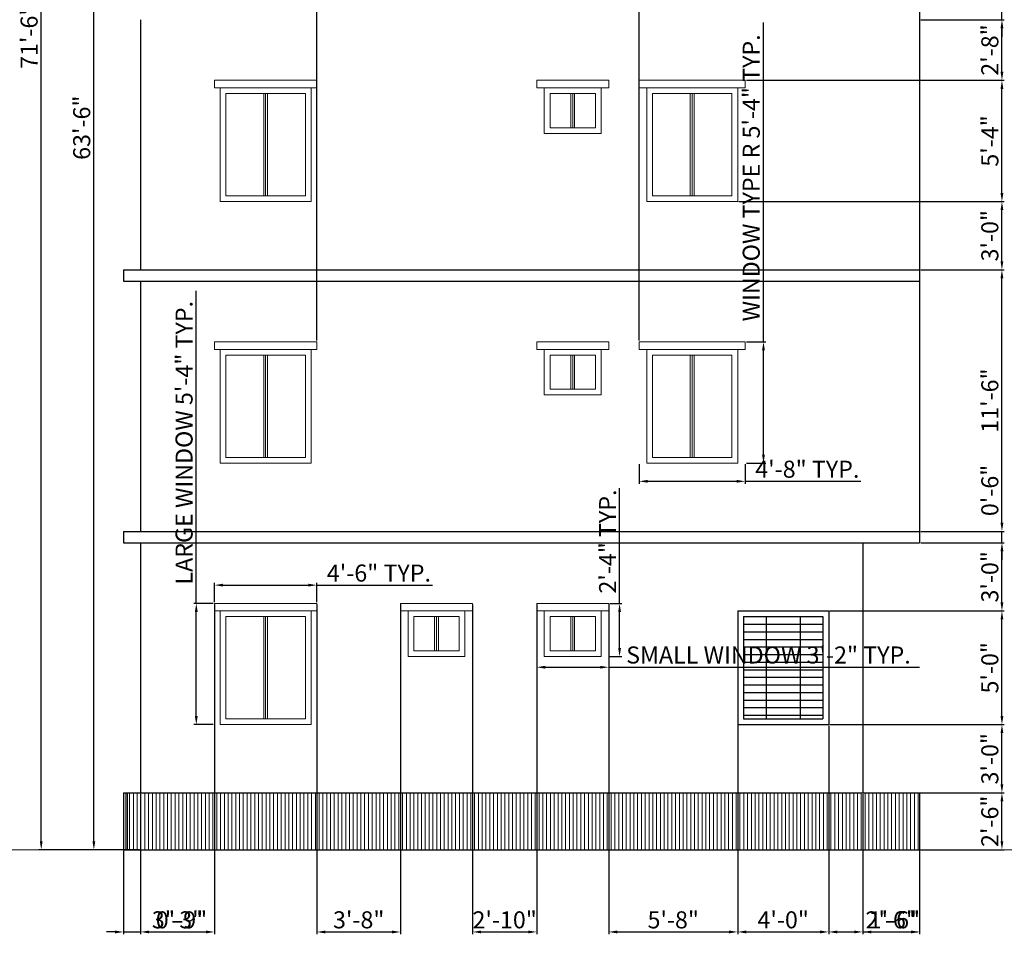
# Model space of a CAD drawing. Units: inches. Extents: x 1692 to 2762, y 798 to 1757.
# Tile 1 of 4: x 1692 to 2211, y 800 to 1282. Entities that reach past the tile are written whole.
import ezdxf

# ---------------------------------------------------------------- set-up
doc = ezdxf.new("R2010")
doc.units = ezdxf.units.IN
for name, color, linetype, lineweight in [('A-ANNO-DIMS', 2, 'Continuous', 18), ('A-CONS', 9, 'Continuous', 13), ('A-ELEV', 7, 'Continuous', 25), ('A-ELEV-PATT', 8, 'Continuous', 13), ('A-GLAZ', 4, 'Continuous', 18)]:
    doc.layers.add(name, color=color, linetype=linetype, lineweight=lineweight)
doc.styles.get("Standard").update_dxf_attribs({"font": 'arial.ttf'})
doc.dimstyles.new('ISO-25', dxfattribs={"dimtxt": 9, "dimasz": 4.5, "dimexe": 1.25, "dimexo": 0.625, "dimtad": 1, "dimdec": 0, "dimlunit": 3, "dimtxsty": 'Standard', "dimcen": 2.5, "dimadec": 0, "dimazin": 0, "dimtfac": 1, "dimtdec": 0, "dimtmove": 0, "dimatfit": 3, "dimfxl": 1, "dimarcsym": 0})

# ---------------------------------------------------------------- blocks, each defined once
blk = doc.blocks.new('*D12')
at = {"layer": 'A-ANNO-DIMS', "color": 0, "lineweight": -2, "transparency": 16777216}
for p, q in [((1755.16, 1606.43), (1729.9, 1606.43)), ((1731.15, 848.93), (1731.15, 1601.93)), ((1755.16, 844.43), (1729.9, 844.43))]:
    blk.add_line(p, q, dxfattribs=at)
at = {"layer": 'A-ANNO-DIMS', "color": 0, "lineweight": 0, "transparency": 16777216}
for points in [[(1730.4, 1601.93), (1731.9, 1601.93), (1731.15, 1606.43)], [(1730.4, 848.93), (1731.9, 848.93), (1731.15, 844.43)]]:
    blk.add_solid(points, dxfattribs=at)
at = {"layer": 'Defpoints', "color": 0, "lineweight": 0, "transparency": 16777216}
for p in [(1731.15, 1606.43), (1755.78, 1606.43), (1755.78, 844.43)]:
    blk.add_point(p, dxfattribs=at)
at = {"layer": 'A-ANNO-DIMS', "color": 0, "transparency": 16777216, "insert": (1725.92, 1225.43), "char_height": 9, "attachment_point": 5, "rotation": 90}
blk.add_mtext('63\'-6"', dxfattribs=at)
blk = doc.blocks.new('WIN-ELEV-L')
for p, q in [((1794.78, 974.43), (1848.78, 974.43)), ((1794.78, 974.43), (1794.78, 970.43)), ((1797.78, 974.43), (1794.78, 974.43)), ((1845.78, 974.43), (1848.78, 974.43)), ((1848.78, 974.43), (1848.78, 970.43)), ((1794.78, 970.43), (1848.78, 970.43)), ((1797.78, 970.43), (1797.78, 910.43)), ((1800.78, 967.43), (1842.78, 967.43)), ((1800.78, 967.43), (1800.78, 913.43)), ((1820.78, 967.43), (1820.78, 913.43)), ((1821.78, 967.43), (1821.78, 913.43)), ((1822.78, 967.43), (1822.78, 913.43)), ((1842.78, 967.43), (1842.78, 913.43)), ((1845.78, 970.43), (1845.78, 910.43)), ((1797.78, 910.43), (1845.78, 910.43)), ((1797.78, 910.43), (1845.78, 910.43)), ((1800.78, 913.43), (1842.78, 913.43))]:
    blk.add_line(p, q)
blk = doc.blocks.new('WIN-ELEV-R')
for p, q in [((2018.78, 1112.43), (2074.78, 1112.43)), ((2018.78, 1112.43), (2018.78, 1108.43)), ((2074.78, 1112.43), (2074.78, 1108.43)), ((2018.78, 1108.43), (2074.78, 1108.43)), ((2022.78, 1108.43), (2022.78, 1048.43)), ((2070.78, 1108.43), (2070.78, 1048.43)), ((2025.78, 1105.43), (2067.78, 1105.43)), ((2025.78, 1105.43), (2025.78, 1051.43)), ((2045.78, 1105.43), (2045.78, 1051.43)), ((2046.78, 1105.43), (2046.78, 1051.43)), ((2047.78, 1105.43), (2047.78, 1051.43)), ((2067.78, 1105.43), (2067.78, 1051.43)), ((2025.78, 1051.43), (2067.78, 1051.43)), ((2022.78, 1048.43), (2070.78, 1048.43))]:
    blk.add_line(p, q)
blk = doc.blocks.new('WIN-ELEV-S')
for p, q in [((1964.78, 974.43), (2002.78, 974.43)), ((1964.78, 974.43), (1964.78, 970.43)), ((2002.78, 974.43), (2002.78, 970.43)), ((1964.78, 970.43), (2002.78, 970.43)), ((1968.78, 970.43), (1968.78, 946.43)), ((1971.78, 967.43), (1995.78, 967.43)), ((1971.78, 967.43), (1971.78, 949.43)), ((1982.78, 967.43), (1982.78, 949.43)), ((1983.78, 967.43), (1983.78, 949.43)), ((1984.78, 967.43), (1984.78, 949.43)), ((1995.78, 967.43), (1995.78, 949.43)), ((1998.78, 970.43), (1998.78, 946.43)), ((1968.78, 946.43), (1998.78, 946.43)), ((1971.78, 949.43), (1995.78, 949.43))]:
    blk.add_line(p, q)
blk = doc.blocks.new('*D18')
at = {"layer": 'A-ANNO-DIMS', "color": 0, "lineweight": -2, "transparency": 16777216}
for p, q in [((1964.78, 945.81), (1964.78, 939.48)), ((2002.78, 945.81), (2002.78, 939.48)), ((1969.28, 940.73), (1998.28, 940.73)), ((2002.78, 940.73), (2166.73, 940.73))]:
    blk.add_line(p, q, dxfattribs=at)
at = {"layer": 'A-ANNO-DIMS', "color": 0, "lineweight": 0, "transparency": 16777216}
for points in [[(1969.28, 941.48), (1969.28, 939.98), (1964.78, 940.73)], [(1998.28, 941.48), (1998.28, 939.98), (2002.78, 940.73)]]:
    blk.add_solid(points, dxfattribs=at)
at = {"layer": 'Defpoints', "color": 0, "lineweight": 0, "transparency": 16777216}
for p in [(1964.78, 946.43), (2002.78, 946.43), (2002.78, 940.73)]:
    blk.add_point(p, dxfattribs=at)
at = {"layer": 'A-ANNO-DIMS', "color": 0, "transparency": 16777216, "insert": (2087.01, 946.02), "char_height": 9, "attachment_point": 5}
blk.add_mtext('SMALL WINDOW 3\'-2" TYP.', dxfattribs=at)
blk = doc.blocks.new('*D19')
at = {"layer": 'A-ANNO-DIMS', "color": 0, "lineweight": -2, "transparency": 16777216}
for p, q in [((2008.48, 974.43), (2008.48, 1035.2)), ((2003.41, 974.43), (2009.73, 974.43)), ((2008.48, 950.93), (2008.48, 969.93)), ((2003.41, 946.43), (2009.73, 946.43))]:
    blk.add_line(p, q, dxfattribs=at)
at = {"layer": 'A-ANNO-DIMS', "color": 0, "lineweight": 0, "transparency": 16777216}
for points in [[(2007.73, 969.93), (2009.23, 969.93), (2008.48, 974.43)], [(2007.73, 950.93), (2009.23, 950.93), (2008.48, 946.43)]]:
    blk.add_solid(points, dxfattribs=at)
at = {"layer": 'Defpoints', "color": 0, "lineweight": 0, "transparency": 16777216}
for p in [(2002.78, 974.43), (2008.48, 974.43), (2002.78, 946.43)]:
    blk.add_point(p, dxfattribs=at)
at = {"layer": 'A-ANNO-DIMS', "color": 0, "transparency": 16777216, "insert": (2003.33, 1007.06), "char_height": 9, "attachment_point": 5, "rotation": 90}
blk.add_mtext('2\'-4" TYP.', dxfattribs=at)
blk = doc.blocks.new('*D20')
at = {"layer": 'A-ANNO-DIMS', "color": 0, "lineweight": -2, "transparency": 16777216}
for p, q in [((1785.18, 974.43), (1785.18, 1139.42)), ((1794.16, 974.43), (1783.93, 974.43)), ((1785.18, 914.93), (1785.18, 969.93)), ((1794.16, 910.43), (1783.93, 910.43))]:
    blk.add_line(p, q, dxfattribs=at)
at = {"layer": 'A-ANNO-DIMS', "color": 0, "lineweight": 0, "transparency": 16777216}
for points in [[(1784.43, 969.93), (1785.93, 969.93), (1785.18, 974.43)], [(1784.43, 914.93), (1785.93, 914.93), (1785.18, 910.43)]]:
    blk.add_solid(points, dxfattribs=at)
at = {"layer": 'Defpoints', "color": 0, "lineweight": 0, "transparency": 16777216}
for p in [(1785.18, 974.43), (1794.78, 974.43), (1794.78, 910.43)]:
    blk.add_point(p, dxfattribs=at)
at = {"layer": 'A-ANNO-DIMS', "color": 0, "transparency": 16777216, "insert": (1779.9, 1059.18), "char_height": 9, "attachment_point": 5, "rotation": 90}
blk.add_mtext('LARGE WINDOW 5\'-4" TYP.', dxfattribs=at)
blk = doc.blocks.new('*D21')
at = {"layer": 'A-ANNO-DIMS', "color": 0, "lineweight": -2, "transparency": 16777216}
for p, q in [((1794.78, 975.06), (1794.78, 985.28)), ((1799.28, 984.03), (1844.28, 984.03)), ((1848.78, 975.06), (1848.78, 985.28)), ((1848.78, 984.03), (1909.75, 984.03))]:
    blk.add_line(p, q, dxfattribs=at)
at = {"layer": 'A-ANNO-DIMS', "color": 0, "lineweight": 0, "transparency": 16777216}
for points in [[(1799.28, 984.78), (1799.28, 983.28), (1794.78, 984.03)], [(1844.28, 984.78), (1844.28, 983.28), (1848.78, 984.03)]]:
    blk.add_solid(points, dxfattribs=at)
at = {"layer": 'Defpoints', "color": 0, "lineweight": 0, "transparency": 16777216}
for p in [(1848.78, 984.03), (1794.78, 974.43), (1848.78, 974.43)]:
    blk.add_point(p, dxfattribs=at)
at = {"layer": 'A-ANNO-DIMS', "color": 0, "transparency": 16777216, "insert": (1881.52, 989.25), "char_height": 9, "attachment_point": 5}
blk.add_mtext('4\'-6" TYP.', dxfattribs=at)
blk = doc.blocks.new('*D22')
at = {"layer": 'A-ANNO-DIMS', "color": 0, "lineweight": -2, "transparency": 16777216}
for p, q in [((2084.38, 1112.43), (2084.38, 1280.97)), ((2075.41, 1112.43), (2085.63, 1112.43)), ((2084.38, 1052.93), (2084.38, 1107.93)), ((2075.41, 1048.43), (2085.63, 1048.43))]:
    blk.add_line(p, q, dxfattribs=at)
at = {"layer": 'A-ANNO-DIMS', "color": 0, "lineweight": 0, "transparency": 16777216}
for points in [[(2083.63, 1107.93), (2085.13, 1107.93), (2084.38, 1112.43)], [(2083.63, 1052.93), (2085.13, 1052.93), (2084.38, 1048.43)]]:
    blk.add_solid(points, dxfattribs=at)
at = {"layer": 'Defpoints', "color": 0, "lineweight": 0, "transparency": 16777216}
for p in [(2074.78, 1112.43), (2084.38, 1112.43), (2074.78, 1048.43)]:
    blk.add_point(p, dxfattribs=at)
at = {"layer": 'A-ANNO-DIMS', "color": 0, "transparency": 16777216, "insert": (2079.1, 1198.95), "char_height": 9, "attachment_point": 5, "rotation": 90}
blk.add_mtext('WINDOW TYPE R 5\'-4" TYP.', dxfattribs=at)
blk = doc.blocks.new('*D23')
at = {"layer": 'A-ANNO-DIMS', "color": 0, "lineweight": -2, "transparency": 16777216}
for p, q in [((2018.78, 1047.81), (2018.78, 1037.58)), ((2074.78, 1047.81), (2074.78, 1037.58)), ((2023.28, 1038.83), (2070.28, 1038.83)), ((2074.78, 1038.83), (2135.75, 1038.83))]:
    blk.add_line(p, q, dxfattribs=at)
at = {"layer": 'A-ANNO-DIMS', "color": 0, "lineweight": 0, "transparency": 16777216}
for points in [[(2023.28, 1039.58), (2023.28, 1038.08), (2018.78, 1038.83)], [(2070.28, 1039.58), (2070.28, 1038.08), (2074.78, 1038.83)]]:
    blk.add_solid(points, dxfattribs=at)
at = {"layer": 'Defpoints', "color": 0, "lineweight": 0, "transparency": 16777216}
for p in [(2018.78, 1048.43), (2074.78, 1048.43), (2074.78, 1038.83)]:
    blk.add_point(p, dxfattribs=at)
at = {"layer": 'A-ANNO-DIMS', "color": 0, "transparency": 16777216, "insert": (2107.52, 1044.05), "char_height": 9, "attachment_point": 5}
blk.add_mtext('4\'-8" TYP.', dxfattribs=at)
blk = doc.blocks.new('*D24')
at = {"layer": 'A-ANNO-DIMS', "color": 0, "lineweight": -2, "transparency": 16777216}
for p, q in [((1950.16, 1702.43), (1702.13, 1702.43)), ((1703.38, 848.93), (1703.38, 1697.93)), ((1746.16, 844.43), (1702.13, 844.43))]:
    blk.add_line(p, q, dxfattribs=at)
at = {"layer": 'A-ANNO-DIMS', "color": 0, "lineweight": 0, "transparency": 16777216}
for points in [[(1702.63, 1697.93), (1704.13, 1697.93), (1703.38, 1702.43)], [(1702.63, 848.93), (1704.13, 848.93), (1703.38, 844.43)]]:
    blk.add_solid(points, dxfattribs=at)
at = {"layer": 'Defpoints', "color": 0, "lineweight": 0, "transparency": 16777216}
for p in [(1703.38, 1702.43), (1950.78, 1702.43), (1746.78, 844.43)]:
    blk.add_point(p, dxfattribs=at)
at = {"layer": 'A-ANNO-DIMS', "color": 0, "transparency": 16777216, "insert": (1698.16, 1273.43), "char_height": 9, "attachment_point": 5, "rotation": 90}
blk.add_mtext('71\'-6"', dxfattribs=at)
blk = doc.blocks.new('*D25')
at = {"layer": 'A-ANNO-DIMS', "color": 0, "lineweight": -2, "transparency": 16777216}
for p, q in [((2167.41, 874.43), (2211.43, 874.43)), ((2210.18, 848.93), (2210.18, 869.93)), ((2167.41, 844.43), (2211.43, 844.43))]:
    blk.add_line(p, q, dxfattribs=at)
at = {"layer": 'A-ANNO-DIMS', "color": 0, "lineweight": 0, "transparency": 16777216}
for points in [[(2209.43, 869.93), (2210.93, 869.93), (2210.18, 874.43)], [(2209.43, 848.93), (2210.93, 848.93), (2210.18, 844.43)]]:
    blk.add_solid(points, dxfattribs=at)
at = {"layer": 'Defpoints', "color": 0, "lineweight": 0, "transparency": 16777216}
for p in [(2166.78, 874.43), (2210.18, 874.43), (2166.78, 844.43)]:
    blk.add_point(p, dxfattribs=at)
at = {"layer": 'A-ANNO-DIMS', "color": 0, "transparency": 16777216, "insert": (2204.96, 859.43), "char_height": 9, "attachment_point": 5, "rotation": 90}
blk.add_mtext('2\'-6"', dxfattribs=at)
blk = doc.blocks.new('*D26')
at = {"layer": 'A-ANNO-DIMS', "color": 0, "lineweight": -2, "transparency": 16777216}
for p, q in [((2119.41, 910.43), (2211.43, 910.43)), ((2210.18, 878.93), (2210.18, 905.93)), ((2137.41, 874.43), (2211.43, 874.43))]:
    blk.add_line(p, q, dxfattribs=at)
at = {"layer": 'A-ANNO-DIMS', "color": 0, "lineweight": 0, "transparency": 16777216}
for points in [[(2209.43, 905.93), (2210.93, 905.93), (2210.18, 910.43)], [(2209.43, 878.93), (2210.93, 878.93), (2210.18, 874.43)]]:
    blk.add_solid(points, dxfattribs=at)
at = {"layer": 'Defpoints', "color": 0, "lineweight": 0, "transparency": 16777216}
for p in [(2118.78, 910.43), (2210.18, 910.43), (2136.78, 874.43)]:
    blk.add_point(p, dxfattribs=at)
at = {"layer": 'A-ANNO-DIMS', "color": 0, "transparency": 16777216, "insert": (2204.96, 892.43), "char_height": 9, "attachment_point": 5, "rotation": 90}
blk.add_mtext('3\'-0"', dxfattribs=at)
blk = doc.blocks.new('*D27')
at = {"layer": 'A-ANNO-DIMS', "color": 0, "lineweight": -2, "transparency": 16777216}
for p, q in [((2119.41, 970.43), (2211.43, 970.43)), ((2210.18, 914.93), (2210.18, 965.93)), ((2119.41, 910.43), (2211.43, 910.43))]:
    blk.add_line(p, q, dxfattribs=at)
at = {"layer": 'A-ANNO-DIMS', "color": 0, "lineweight": 0, "transparency": 16777216}
for points in [[(2209.43, 965.93), (2210.93, 965.93), (2210.18, 970.43)], [(2209.43, 914.93), (2210.93, 914.93), (2210.18, 910.43)]]:
    blk.add_solid(points, dxfattribs=at)
at = {"layer": 'Defpoints', "color": 0, "lineweight": 0, "transparency": 16777216}
for p in [(2118.78, 970.43), (2210.18, 970.43), (2118.78, 910.43)]:
    blk.add_point(p, dxfattribs=at)
at = {"layer": 'A-ANNO-DIMS', "color": 0, "transparency": 16777216, "insert": (2204.96, 940.43), "char_height": 9, "attachment_point": 5, "rotation": 90}
blk.add_mtext('5\'-0"', dxfattribs=at)
blk = doc.blocks.new('*D28')
at = {"layer": 'A-ANNO-DIMS', "color": 0, "lineweight": -2, "transparency": 16777216}
for p, q in [((2167.41, 1006.43), (2211.43, 1006.43)), ((2210.18, 974.93), (2210.18, 1001.93)), ((2119.41, 970.43), (2211.43, 970.43))]:
    blk.add_line(p, q, dxfattribs=at)
at = {"layer": 'A-ANNO-DIMS', "color": 0, "lineweight": 0, "transparency": 16777216}
for points in [[(2209.43, 1001.93), (2210.93, 1001.93), (2210.18, 1006.43)], [(2209.43, 974.93), (2210.93, 974.93), (2210.18, 970.43)]]:
    blk.add_solid(points, dxfattribs=at)
at = {"layer": 'Defpoints', "color": 0, "lineweight": 0, "transparency": 16777216}
for p in [(2166.78, 1006.43), (2210.18, 1006.43), (2118.78, 970.43)]:
    blk.add_point(p, dxfattribs=at)
at = {"layer": 'A-ANNO-DIMS', "color": 0, "transparency": 16777216, "insert": (2204.96, 988.43), "char_height": 9, "attachment_point": 5, "rotation": 90}
blk.add_mtext('3\'-0"', dxfattribs=at)
blk = doc.blocks.new('*D29')
at = {"layer": 'A-ANNO-DIMS', "color": 0, "lineweight": -2, "transparency": 16777216}
for p, q in [((2210.18, 1016.93), (2210.18, 1046.61)), ((2167.41, 1012.43), (2211.43, 1012.43)), ((2210.18, 1006.43), (2210.18, 1012.43)), ((2167.41, 1006.43), (2211.43, 1006.43)), ((2210.18, 1001.93), (2210.18, 997.43))]:
    blk.add_line(p, q, dxfattribs=at)
at = {"layer": 'A-ANNO-DIMS', "color": 0, "lineweight": 0, "transparency": 16777216}
for points in [[(2209.43, 1016.93), (2210.93, 1016.93), (2210.18, 1012.43)], [(2209.43, 1001.93), (2210.93, 1001.93), (2210.18, 1006.43)]]:
    blk.add_solid(points, dxfattribs=at)
at = {"layer": 'Defpoints', "color": 0, "lineweight": 0, "transparency": 16777216}
for p in [(2166.78, 1012.43), (2210.18, 1012.43), (2166.78, 1006.43)]:
    blk.add_point(p, dxfattribs=at)
at = {"layer": 'A-ANNO-DIMS', "color": 0, "transparency": 16777216, "insert": (2204.96, 1034.02), "char_height": 9, "attachment_point": 5, "rotation": 90}
blk.add_mtext('0\'-6"', dxfattribs=at)
blk = doc.blocks.new('*D30')
at = {"layer": 'A-ANNO-DIMS', "color": 0, "lineweight": -2, "transparency": 16777216}
for p, q in [((2167.41, 1150.43), (2211.43, 1150.43)), ((2210.18, 1016.93), (2210.18, 1145.93)), ((2167.41, 1012.43), (2211.43, 1012.43))]:
    blk.add_line(p, q, dxfattribs=at)
at = {"layer": 'A-ANNO-DIMS', "color": 0, "lineweight": 0, "transparency": 16777216}
for points in [[(2209.43, 1145.93), (2210.93, 1145.93), (2210.18, 1150.43)], [(2209.43, 1016.93), (2210.93, 1016.93), (2210.18, 1012.43)]]:
    blk.add_solid(points, dxfattribs=at)
at = {"layer": 'Defpoints', "color": 0, "lineweight": 0, "transparency": 16777216}
for p in [(2166.78, 1150.43), (2210.18, 1150.43), (2166.78, 1012.43)]:
    blk.add_point(p, dxfattribs=at)
at = {"layer": 'A-ANNO-DIMS', "color": 0, "transparency": 16777216, "insert": (2204.96, 1081.43), "char_height": 9, "attachment_point": 5, "rotation": 90}
blk.add_mtext('11\'-6"', dxfattribs=at)
blk = doc.blocks.new('*D31')
at = {"layer": 'A-ANNO-DIMS', "color": 0, "lineweight": -2, "transparency": 16777216}
for p, q in [((2071.41, 1186.43), (2211.43, 1186.43)), ((2210.18, 1154.93), (2210.18, 1181.93)), ((2167.41, 1150.43), (2211.43, 1150.43))]:
    blk.add_line(p, q, dxfattribs=at)
at = {"layer": 'A-ANNO-DIMS', "color": 0, "lineweight": 0, "transparency": 16777216}
for points in [[(2209.43, 1181.93), (2210.93, 1181.93), (2210.18, 1186.43)], [(2209.43, 1154.93), (2210.93, 1154.93), (2210.18, 1150.43)]]:
    blk.add_solid(points, dxfattribs=at)
at = {"layer": 'Defpoints', "color": 0, "lineweight": 0, "transparency": 16777216}
for p in [(2070.78, 1186.43), (2210.18, 1186.43), (2166.78, 1150.43)]:
    blk.add_point(p, dxfattribs=at)
at = {"layer": 'A-ANNO-DIMS', "color": 0, "transparency": 16777216, "insert": (2204.96, 1168.43), "char_height": 9, "attachment_point": 5, "rotation": 90}
blk.add_mtext('3\'-0"', dxfattribs=at)
blk = doc.blocks.new('*D32')
at = {"layer": 'A-ANNO-DIMS', "color": 0, "lineweight": -2, "transparency": 16777216}
for p, q in [((2075.41, 1250.43), (2211.43, 1250.43)), ((2210.18, 1190.93), (2210.18, 1245.93)), ((2071.41, 1186.43), (2211.43, 1186.43))]:
    blk.add_line(p, q, dxfattribs=at)
at = {"layer": 'A-ANNO-DIMS', "color": 0, "lineweight": 0, "transparency": 16777216}
for points in [[(2209.43, 1245.93), (2210.93, 1245.93), (2210.18, 1250.43)], [(2209.43, 1190.93), (2210.93, 1190.93), (2210.18, 1186.43)]]:
    blk.add_solid(points, dxfattribs=at)
at = {"layer": 'Defpoints', "color": 0, "lineweight": 0, "transparency": 16777216}
for p in [(2074.78, 1250.43), (2210.18, 1250.43), (2070.78, 1186.43)]:
    blk.add_point(p, dxfattribs=at)
at = {"layer": 'A-ANNO-DIMS', "color": 0, "transparency": 16777216, "insert": (2204.98, 1218.43), "char_height": 9, "attachment_point": 5, "rotation": 90}
blk.add_mtext('5\'-4"', dxfattribs=at)
blk = doc.blocks.new('*D33')
at = {"layer": 'A-ANNO-DIMS', "color": 0, "lineweight": -2, "transparency": 16777216}
for p, q in [((2167.41, 1282.43), (2211.43, 1282.43)), ((2210.18, 1254.93), (2210.18, 1277.93)), ((2075.41, 1250.43), (2211.43, 1250.43))]:
    blk.add_line(p, q, dxfattribs=at)
at = {"layer": 'A-ANNO-DIMS', "color": 0, "lineweight": 0, "transparency": 16777216}
for points in [[(2209.43, 1277.93), (2210.93, 1277.93), (2210.18, 1282.43)], [(2209.43, 1254.93), (2210.93, 1254.93), (2210.18, 1250.43)]]:
    blk.add_solid(points, dxfattribs=at)
at = {"layer": 'Defpoints', "color": 0, "lineweight": 0, "transparency": 16777216}
for p in [(2166.78, 1282.43), (2210.18, 1282.43), (2074.78, 1250.43)]:
    blk.add_point(p, dxfattribs=at)
at = {"layer": 'A-ANNO-DIMS', "color": 0, "transparency": 16777216, "insert": (2204.96, 1266.43), "char_height": 9, "attachment_point": 5, "rotation": 90}
blk.add_mtext('2\'-8"', dxfattribs=at)
blk = doc.blocks.new('*D34')
at = {"layer": 'A-ANNO-DIMS', "color": 0, "lineweight": -2, "transparency": 16777216}
for p, q in [((2210.18, 1292.93), (2210.18, 1322.61)), ((2167.41, 1288.43), (2211.43, 1288.43)), ((2210.18, 1282.43), (2210.18, 1288.43)), ((2167.41, 1282.43), (2211.43, 1282.43)), ((2210.18, 1277.93), (2210.18, 1273.43))]:
    blk.add_line(p, q, dxfattribs=at)
at = {"layer": 'A-ANNO-DIMS', "color": 0, "lineweight": 0, "transparency": 16777216}
for points in [[(2209.43, 1292.93), (2210.93, 1292.93), (2210.18, 1288.43)], [(2209.43, 1277.93), (2210.93, 1277.93), (2210.18, 1282.43)]]:
    blk.add_solid(points, dxfattribs=at)
at = {"layer": 'Defpoints', "color": 0, "lineweight": 0, "transparency": 16777216}
for p in [(2166.78, 1288.43), (2210.18, 1288.43), (2166.78, 1282.43)]:
    blk.add_point(p, dxfattribs=at)
at = {"layer": 'A-ANNO-DIMS', "color": 0, "transparency": 16777216, "insert": (2204.96, 1310.02), "char_height": 9, "attachment_point": 5, "rotation": 90}
blk.add_mtext('0\'-6"', dxfattribs=at)
blk = doc.blocks.new('*D39')
at = {"layer": 'A-ANNO-DIMS', "color": 0, "lineweight": -2, "transparency": 16777216}
for p, q in [((1755.78, 873.81), (1755.78, 799.78)), ((1746.78, 843.81), (1746.78, 799.78)), ((1742.28, 801.03), (1737.78, 801.03)), ((1746.78, 801.03), (1755.78, 801.03)), ((1760.28, 801.03), (1789.95, 801.03))]:
    blk.add_line(p, q, dxfattribs=at)
at = {"layer": 'A-ANNO-DIMS', "color": 0, "lineweight": 0, "transparency": 16777216}
for points in [[(1742.28, 801.78), (1742.28, 800.28), (1746.78, 801.03)], [(1760.28, 801.78), (1760.28, 800.28), (1755.78, 801.03)]]:
    blk.add_solid(points, dxfattribs=at)
at = {"layer": 'Defpoints', "color": 0, "lineweight": 0, "transparency": 16777216}
for p in [(1755.78, 874.43), (1746.78, 844.43), (1755.78, 801.03)]:
    blk.add_point(p, dxfattribs=at)
at = {"layer": 'A-ANNO-DIMS', "color": 0, "transparency": 16777216, "insert": (1777.37, 806.25), "char_height": 9, "attachment_point": 5}
blk.add_mtext('0\'-9"', dxfattribs=at)
blk = doc.blocks.new('*D40')
at = {"layer": 'A-ANNO-DIMS', "color": 0, "lineweight": -2, "transparency": 16777216}
for p, q in [((1794.78, 973.81), (1794.78, 799.78)), ((1755.78, 873.81), (1755.78, 799.78)), ((1760.28, 801.03), (1790.28, 801.03))]:
    blk.add_line(p, q, dxfattribs=at)
at = {"layer": 'A-ANNO-DIMS', "color": 0, "lineweight": 0, "transparency": 16777216}
for points in [[(1760.28, 801.78), (1760.28, 800.28), (1755.78, 801.03)], [(1790.28, 801.78), (1790.28, 800.28), (1794.78, 801.03)]]:
    blk.add_solid(points, dxfattribs=at)
at = {"layer": 'Defpoints', "color": 0, "lineweight": 0, "transparency": 16777216}
for p in [(1794.78, 974.43), (1755.78, 874.43), (1794.78, 801.03)]:
    blk.add_point(p, dxfattribs=at)
at = {"layer": 'A-ANNO-DIMS', "color": 0, "transparency": 16777216, "insert": (1775.28, 806.26), "char_height": 9, "attachment_point": 5}
blk.add_mtext('3\'-3"', dxfattribs=at)
blk = doc.blocks.new('*D41')
at = {"layer": 'A-ANNO-DIMS', "color": 0, "lineweight": -2, "transparency": 16777216}
for p, q in [((1848.78, 973.81), (1848.78, 799.78)), ((1892.93, 973.81), (1892.93, 799.78)), ((1853.28, 801.03), (1888.43, 801.03))]:
    blk.add_line(p, q, dxfattribs=at)
at = {"layer": 'A-ANNO-DIMS', "color": 0, "lineweight": 0, "transparency": 16777216}
for points in [[(1853.28, 801.78), (1853.28, 800.28), (1848.78, 801.03)], [(1888.43, 801.78), (1888.43, 800.28), (1892.93, 801.03)]]:
    blk.add_solid(points, dxfattribs=at)
at = {"layer": 'Defpoints', "color": 0, "lineweight": 0, "transparency": 16777216}
for p in [(1848.78, 974.43), (1892.93, 974.43), (1892.93, 801.03)]:
    blk.add_point(p, dxfattribs=at)
at = {"layer": 'A-ANNO-DIMS', "color": 0, "transparency": 16777216, "insert": (1870.86, 806.26), "char_height": 9, "attachment_point": 5}
blk.add_mtext('3\'-8"', dxfattribs=at)
blk = doc.blocks.new('*D42')
at = {"layer": 'A-ANNO-DIMS', "color": 0, "lineweight": -2, "transparency": 16777216}
for p, q in [((1930.93, 973.81), (1930.93, 799.78)), ((1964.78, 973.81), (1964.78, 799.78)), ((1935.43, 801.03), (1960.28, 801.03))]:
    blk.add_line(p, q, dxfattribs=at)
at = {"layer": 'A-ANNO-DIMS', "color": 0, "lineweight": 0, "transparency": 16777216}
for points in [[(1935.43, 801.78), (1935.43, 800.28), (1930.93, 801.03)], [(1960.28, 801.78), (1960.28, 800.28), (1964.78, 801.03)]]:
    blk.add_solid(points, dxfattribs=at)
at = {"layer": 'Defpoints', "color": 0, "lineweight": 0, "transparency": 16777216}
for p in [(1930.93, 974.43), (1964.78, 974.43), (1964.78, 801.03)]:
    blk.add_point(p, dxfattribs=at)
at = {"layer": 'A-ANNO-DIMS', "color": 0, "transparency": 16777216, "insert": (1947.86, 806.25), "char_height": 9, "attachment_point": 5}
blk.add_mtext('2\'-10"', dxfattribs=at)
blk = doc.blocks.new('*D43')
at = {"layer": 'A-ANNO-DIMS', "color": 0, "lineweight": -2, "transparency": 16777216}
for p, q in [((2002.78, 973.81), (2002.78, 799.78)), ((2070.78, 969.81), (2070.78, 799.78)), ((2007.28, 801.03), (2066.28, 801.03))]:
    blk.add_line(p, q, dxfattribs=at)
at = {"layer": 'A-ANNO-DIMS', "color": 0, "lineweight": 0, "transparency": 16777216}
for points in [[(2007.28, 801.78), (2007.28, 800.28), (2002.78, 801.03)], [(2066.28, 801.78), (2066.28, 800.28), (2070.78, 801.03)]]:
    blk.add_solid(points, dxfattribs=at)
at = {"layer": 'Defpoints', "color": 0, "lineweight": 0, "transparency": 16777216}
for p in [(2002.78, 974.43), (2070.78, 970.43), (2070.78, 801.03)]:
    blk.add_point(p, dxfattribs=at)
at = {"layer": 'A-ANNO-DIMS', "color": 0, "transparency": 16777216, "insert": (2036.78, 806.25), "char_height": 9, "attachment_point": 5}
blk.add_mtext('5\'-8"', dxfattribs=at)
blk = doc.blocks.new('*D44')
at = {"layer": 'A-ANNO-DIMS', "color": 0, "lineweight": -2, "transparency": 16777216}
for p, q in [((2070.78, 909.81), (2070.78, 799.78)), ((2118.78, 909.81), (2118.78, 799.78)), ((2075.28, 801.03), (2114.28, 801.03))]:
    blk.add_line(p, q, dxfattribs=at)
at = {"layer": 'A-ANNO-DIMS', "color": 0, "lineweight": 0, "transparency": 16777216}
for points in [[(2075.28, 801.78), (2075.28, 800.28), (2070.78, 801.03)], [(2114.28, 801.78), (2114.28, 800.28), (2118.78, 801.03)]]:
    blk.add_solid(points, dxfattribs=at)
at = {"layer": 'Defpoints', "color": 0, "lineweight": 0, "transparency": 16777216}
for p in [(2070.78, 910.43), (2118.78, 910.43), (2118.78, 801.03)]:
    blk.add_point(p, dxfattribs=at)
at = {"layer": 'A-ANNO-DIMS', "color": 0, "transparency": 16777216, "insert": (2094.78, 806.25), "char_height": 9, "attachment_point": 5}
blk.add_mtext('4\'-0"', dxfattribs=at)
blk = doc.blocks.new('*D45')
at = {"layer": 'A-ANNO-DIMS', "color": 0, "lineweight": -2, "transparency": 16777216}
for p, q in [((2118.78, 909.81), (2118.78, 799.78)), ((2136.78, 873.81), (2136.78, 799.78)), ((2123.28, 801.03), (2132.28, 801.03)), ((2136.78, 801.03), (2165.61, 801.03))]:
    blk.add_line(p, q, dxfattribs=at)
at = {"layer": 'A-ANNO-DIMS', "color": 0, "lineweight": 0, "transparency": 16777216}
for points in [[(2123.28, 801.78), (2123.28, 800.28), (2118.78, 801.03)], [(2132.28, 801.78), (2132.28, 800.28), (2136.78, 801.03)]]:
    blk.add_solid(points, dxfattribs=at)
at = {"layer": 'Defpoints', "color": 0, "lineweight": 0, "transparency": 16777216}
for p in [(2118.78, 910.43), (2136.78, 874.43), (2136.78, 801.03)]:
    blk.add_point(p, dxfattribs=at)
at = {"layer": 'A-ANNO-DIMS', "color": 0, "transparency": 16777216, "insert": (2153.44, 806.25), "char_height": 9, "attachment_point": 5}
blk.add_mtext('1\'-6"', dxfattribs=at)
blk = doc.blocks.new('*D46')
at = {"layer": 'A-ANNO-DIMS', "color": 0, "lineweight": -2, "transparency": 16777216}
for p, q in [((2136.78, 873.81), (2136.78, 799.78)), ((2166.78, 873.81), (2166.78, 799.78)), ((2141.28, 801.03), (2162.28, 801.03))]:
    blk.add_line(p, q, dxfattribs=at)
at = {"layer": 'A-ANNO-DIMS', "color": 0, "lineweight": 0, "transparency": 16777216}
for points in [[(2141.28, 801.78), (2141.28, 800.28), (2136.78, 801.03)], [(2162.28, 801.78), (2162.28, 800.28), (2166.78, 801.03)]]:
    blk.add_solid(points, dxfattribs=at)
at = {"layer": 'Defpoints', "color": 0, "lineweight": 0, "transparency": 16777216}
for p in [(2136.78, 874.43), (2166.78, 874.43), (2166.78, 801.03)]:
    blk.add_point(p, dxfattribs=at)
at = {"layer": 'A-ANNO-DIMS', "color": 0, "transparency": 16777216, "insert": (2151.78, 806.25), "char_height": 9, "attachment_point": 5}
blk.add_mtext('2\'-6"', dxfattribs=at)
blk = doc.blocks.new('*D47')
at = {"layer": 'A-ANNO-DIMS', "color": 0, "lineweight": -2, "transparency": 16777216}
for p, q in [((1848.78, 1113.06), (1848.78, 1747.08)), ((1853.28, 1745.83), (2014.28, 1745.83)), ((2018.78, 1113.06), (2018.78, 1747.08))]:
    blk.add_line(p, q, dxfattribs=at)
at = {"layer": 'A-ANNO-DIMS', "color": 0, "lineweight": 0, "transparency": 16777216}
for points in [[(1853.28, 1746.58), (1853.28, 1745.08), (1848.78, 1745.83)], [(2014.28, 1746.58), (2014.28, 1745.08), (2018.78, 1745.83)]]:
    blk.add_solid(points, dxfattribs=at)
at = {"layer": 'Defpoints', "color": 0, "lineweight": 0, "transparency": 16777216}
for p in [(2018.78, 1745.83), (1848.78, 1112.43), (2018.78, 1112.43)]:
    blk.add_point(p, dxfattribs=at)
at = {"layer": 'A-ANNO-DIMS', "color": 0, "transparency": 16777216, "insert": (1933.78, 1750.98), "char_height": 9, "attachment_point": 5}
blk.add_mtext('14\'-2"', dxfattribs=at)

msp = doc.modelspace()

# ---------------------------------------------------------------- hatches: boundary and pattern name
at = {"layer": 'A-ELEV-PATT'}
h = msp.add_hatch(dxfattribs=at)
h.set_pattern_fill('ANSI31', color=256, scale=0.629921, angle=45, style=0)
h.paths.add_polyline_path([(1746.78, 844.43), (2166.78, 844.43), (2166.78, 874.43), (1746.78, 874.43)])

# ---------------------------------------------------------------- linework, layer by layer
at = {"layer": 'A-CONS'}
msp.add_xline((2166.78, 844.43), (1, 0), dxfattribs=at)
at = {"layer": 'A-ELEV'}
for p, q in [((2166.78, 1606.43), (2166.78, 1006.43)), ((1755.78, 1282.43), (1755.78, 1150.43)), ((1746.78, 1150.43), (2166.78, 1150.43)), ((1746.78, 1150.43), (1746.78, 1144.43)), ((1746.78, 1144.43), (2166.78, 1144.43)), ((1755.78, 1144.43), (1755.78, 1012.43)), ((1746.78, 1012.43), (2166.78, 1012.43)), ((1746.78, 1012.43), (1746.78, 1006.43)), ((1746.78, 1006.43), (2166.78, 1006.43)), ((1755.78, 1006.43), (1755.78, 874.43)), ((2136.78, 1006.43), (2136.78, 874.43)), ((2070.78, 970.43), (2070.78, 910.43)), ((2070.78, 970.43), (2118.78, 970.43)), ((2073.78, 967.43), (2115.78, 967.43)), ((2073.78, 967.43), (2073.78, 913.43)), ((2085.78, 967.43), (2085.78, 913.43)), ((2103.78, 967.43), (2103.78, 913.43)), ((2115.78, 967.43), (2115.78, 913.43)), ((2118.78, 970.43), (2118.78, 910.43)), ((2073.78, 963.43), (2115.78, 963.43)), ((2073.78, 959.43), (2115.78, 959.43)), ((2073.78, 955.43), (2115.78, 955.43)), ((2073.78, 951.43), (2115.78, 951.43)), ((2073.78, 947.43), (2115.78, 947.43)), ((2073.78, 943.43), (2115.78, 943.43)), ((2073.78, 939.43), (2115.78, 939.43)), ((2073.78, 935.43), (2115.78, 935.43)), ((2073.78, 931.43), (2115.78, 931.43)), ((2073.78, 927.43), (2115.78, 927.43)), ((2073.78, 923.43), (2115.78, 923.43)), ((2073.78, 919.43), (2115.78, 919.43)), ((2073.78, 915.43), (2115.78, 915.43)), ((2070.78, 910.43), (2118.78, 910.43)), ((2073.78, 913.43), (2115.78, 913.43)), ((1746.78, 874.43), (2166.78, 874.43)), ((1746.78, 874.43), (1746.78, 844.43)), ((1746.78, 874.43), (1746.78, 844.43)), ((1746.78, 874.43), (1746.78, 844.43)), ((1748.78, 874.43), (1748.78, 844.43)), ((2166.78, 874.43), (2166.78, 844.43)), ((1746.78, 844.43), (2166.78, 844.43))]:
    msp.add_line(p, q, dxfattribs=at)

# ---------------------------------------------------------------- block references
at = {"layer": 'A-GLAZ'}
for name, p in [('WIN-ELEV-L', (0, 276)), ('WIN-ELEV-S', (0, 276)), ('WIN-ELEV-R', (0, 138)), ('WIN-ELEV-L', (0, 138)), ('WIN-ELEV-S', (0, 138)), ('WIN-ELEV-R', (0, 0)), ('WIN-ELEV-L', (0, 0)), ('WIN-ELEV-S', (-71.85, 0)), ('WIN-ELEV-S', (0, 0))]:
    msp.add_blockref(name, p, dxfattribs=at)

# ---------------------------------------------------------------- dimensions: what is measured, and where the dimension line sits
at = {"layer": 'A-ANNO-DIMS'}
for base, p1, p2, picture, middle in [((2018.78, 1745.83), (1848.78, 1112.43), (2018.78, 1112.43), '*D47', (1933.78, 1750.98)), ((1794.78, 801.03), (1755.78, 874.43), (1794.78, 974.43), '*D40', (1775.28, 806.26)), ((1892.9307, 801.0326), (1848.7805, 974.4326), (1892.9307, 974.4326), '*D41', (1870.8556, 806.2559)), ((1964.7805, 801.0326), (1930.9307, 974.4326), (1964.7805, 974.4326), '*D42', (1947.8556, 806.2528)), ((2070.78, 801.03), (2002.78, 974.43), (2070.78, 970.43), '*D43', (2036.78, 806.25)), ((2118.78, 801.03), (2070.78, 910.43), (2118.78, 910.43), '*D44', (2094.78, 806.25)), ((2136.78, 801.03), (2118.78, 910.43), (2136.78, 874.43), '*D45', (2153.44, 806.25)), ((1755.78, 801.03), (1746.78, 844.43), (1755.78, 874.43), '*D39', (1777.37, 806.25)), ((2166.78, 801.03), (2136.78, 874.43), (2166.78, 874.43), '*D46', (2151.78, 806.25))]:
    dim = msp.add_linear_dim(base=base, p1=p1, p2=p2, dimstyle='ISO-25', override={"dimdec": 1, "dimlfac": 1, "dimrnd": 0, "dimzin": 1, "dimdsep": 46, "dimlunit": 4, "dimfrac": 2}, dxfattribs=at)
    dim.commit()
    dim.dimension.update_dxf_attribs({"geometry": picture, "text_midpoint": middle})
for base, p1, p2, override, picture, middle in [((1703.38, 1702.43), (1746.78, 844.43), (1950.78, 1702.43), {"dimdec": 1, "dimlfac": 1, "dimrnd": 0, "dimzin": 1, "dimdsep": 46, "dimlunit": 4, "dimfrac": 2}, '*D24', (1698.16, 1273.43)), ((1731.15, 1606.43), (1755.78, 844.43), (1755.78, 1606.43), {"dimclrd": 0, "dimclre": 0, "dimclrt": 0}, '*D12', (1725.92, 1225.43)), ((2210.18, 1288.43), (2166.78, 1282.43), (2166.78, 1288.43), {"dimdec": 1, "dimlfac": 1, "dimrnd": 0, "dimzin": 1, "dimdsep": 46, "dimlunit": 4, "dimfrac": 2}, '*D34', (2204.96, 1310.02)), ((2210.18, 1282.43), (2074.78, 1250.43), (2166.78, 1282.43), {"dimdec": 1, "dimlfac": 1, "dimrnd": 0, "dimzin": 1, "dimdsep": 46, "dimlunit": 4, "dimfrac": 2}, '*D33', (2204.96, 1266.43)), ((2210.18, 1250.43), (2070.78, 1186.43), (2074.78, 1250.43), {"dimdec": 1, "dimlfac": 1, "dimrnd": 0, "dimzin": 1, "dimdsep": 46, "dimlunit": 4, "dimfrac": 2}, '*D32', (2204.98, 1218.43)), ((2210.18, 1186.43), (2166.78, 1150.43), (2070.78, 1186.43), {"dimdec": 1, "dimlfac": 1, "dimrnd": 0, "dimzin": 1, "dimdsep": 46, "dimlunit": 4, "dimfrac": 2}, '*D31', (2204.96, 1168.43)), ((2210.18, 1150.43), (2166.78, 1012.43), (2166.78, 1150.43), {"dimdec": 1, "dimlfac": 1, "dimrnd": 0, "dimzin": 1, "dimdsep": 46, "dimlunit": 4, "dimfrac": 2}, '*D30', (2204.96, 1081.43)), ((2210.18, 1012.43), (2166.78, 1006.43), (2166.78, 1012.43), {"dimdec": 1, "dimlfac": 1, "dimrnd": 0, "dimzin": 1, "dimdsep": 46, "dimlunit": 4, "dimfrac": 2}, '*D29', (2204.96, 1034.02)), ((2210.18, 1006.43), (2118.78, 970.43), (2166.78, 1006.43), {"dimdec": 1, "dimlfac": 1, "dimrnd": 0, "dimzin": 1, "dimdsep": 46, "dimlunit": 4, "dimfrac": 2}, '*D28', (2204.96, 988.43)), ((2210.18, 970.43), (2118.78, 910.43), (2118.78, 970.43), {"dimdec": 1, "dimlfac": 1, "dimrnd": 0, "dimzin": 1, "dimdsep": 46, "dimlunit": 4, "dimfrac": 2}, '*D27', (2204.96, 940.43)), ((2210.18, 910.43), (2136.78, 874.43), (2118.78, 910.43), {"dimdec": 1, "dimlfac": 1, "dimrnd": 0, "dimzin": 1, "dimdsep": 46, "dimlunit": 4, "dimfrac": 2}, '*D26', (2204.96, 892.43)), ((2210.18, 874.43), (2166.78, 844.43), (2166.78, 874.43), {"dimdec": 1, "dimlfac": 1, "dimrnd": 0, "dimzin": 1, "dimdsep": 46, "dimlunit": 4, "dimfrac": 2}, '*D25', (2204.96, 859.43))]:
    dim = msp.add_linear_dim(base=base, p1=p1, p2=p2, angle=90, dimstyle='ISO-25', override=override, dxfattribs=at)
    dim.commit()
    dim.dimension.update_dxf_attribs({"geometry": picture, "text_midpoint": middle})
for base, p1, p2, text, picture, middle in [((2084.38, 1112.43), (2074.78, 1048.43), (2074.78, 1112.43), 'WINDOW TYPE R <> TYP.', '*D22', (2079.1, 1198.95)), ((1785.18, 974.43), (1794.78, 910.43), (1794.78, 974.43), 'LARGE WINDOW <> TYP.', '*D20', (1779.9, 1059.18)), ((2008.48, 974.43), (2002.78, 946.43), (2002.78, 974.43), '<> TYP.', '*D19', (2003.33, 1007.06))]:
    dim = msp.add_linear_dim(base=base, p1=p1, p2=p2, angle=90, text=text, dimstyle='ISO-25', override={"dimdec": 1, "dimrnd": 0, "dimzin": 1, "dimlunit": 4, "dimfrac": 2}, dxfattribs=at)
    dim.commit()
    dim.dimension.update_dxf_attribs({"geometry": picture, "text_midpoint": middle})
for base, p1, p2, text, picture, middle in [((2074.78, 1038.83), (2018.78, 1048.43), (2074.78, 1048.43), '<> TYP.', '*D23', (2107.52, 1044.05)), ((1848.78, 984.03), (1794.78, 974.43), (1848.78, 974.43), '<> TYP.', '*D21', (1881.52, 989.25)), ((2002.78, 940.73), (1964.78, 946.43), (2002.78, 946.43), 'SMALL WINDOW <> TYP.', '*D18', (2087.01, 946.02))]:
    dim = msp.add_linear_dim(base=base, p1=p1, p2=p2, text=text, dimstyle='ISO-25', override={"dimdec": 1, "dimrnd": 0, "dimzin": 1, "dimlunit": 4, "dimfrac": 2}, dxfattribs=at)
    dim.commit()
    dim.dimension.update_dxf_attribs({"geometry": picture, "text_midpoint": middle})

doc.saveas('drawing.dxf')
